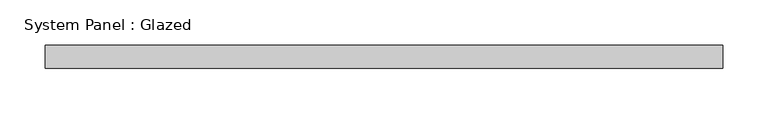
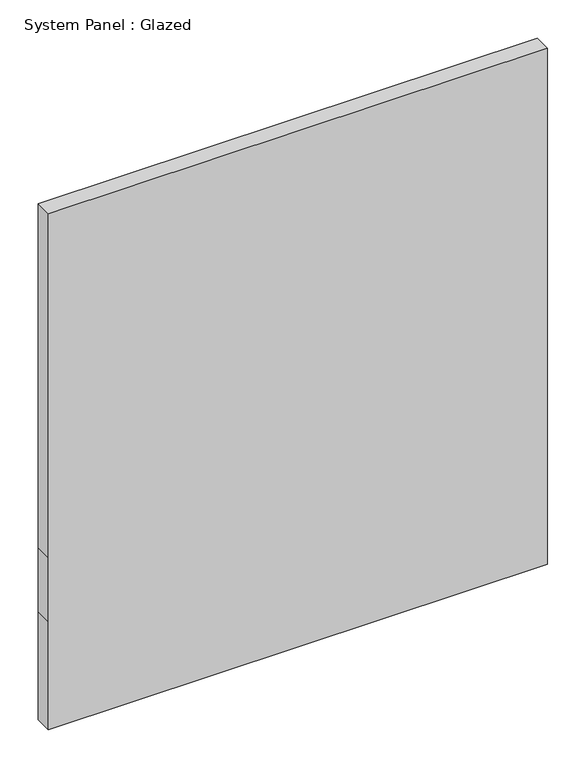
"""IFC4 building model written with IfcOpenShell, lengths in millimetres: plate geometry, System Panel : Glazed."""

from ifc_helpers import new_model, si_unit, frame, origin, place, context, project, spatial, polyline, outline, extrude, source, transform, mapped, element, save


def system_panel_glazed_e6cace74(model_context):
    return source(origin(), model_context, "Body", "SweptSolid", [
        extrude(outline(polyline([(0.0, -374.65), (0.0, 374.65), (171.3165682, 374.65), (272.8498523, 374.65), (818.549557, 374.65), (818.549557, -374.65), (272.8498523, -374.65), (171.3165682, -374.65), (0.0, -374.65)])), frame((0.0, 19.05, 0.0), z_axis=(0.0, 1.0, 0.0), x_axis=(0.0, 0.0, 1.0)), (0.0, 0.0, 1.0), 25.4),
    ])


if __name__ == "__main__":
    model = new_model("IFC4")
    model_context = context("Model", 3, world=origin())
    ifc_project = project(units=[si_unit("LENGTHUNIT", "METRE", prefix="MILLI")], contexts=[model_context])
    site = spatial("IfcSite", under=ifc_project)
    building = spatial("IfcBuilding", under=site)
    placement = place(None, origin())
    system_panel_glazed_shape = system_panel_glazed_e6cace74(model_context)
    element("IfcPlate", 1, ObjectType="System Panel : Glazed", at=placement, inside=building, context=model_context, shape_type="MappedRepresentation", body=[
        mapped(system_panel_glazed_shape, transform((0.0, 0.0, 0.0), x_axis=(1.0, 0.0, 0.0), y_axis=(0.0, 1.0, 0.0), z_axis=(0.0, 0.0, 1.0))),
    ])
    save(model, "model.ifc")

# Revit data of these elements
# Type "System Panel : Glazed"
#   Construction Type Id = "GSP4R"
#   Analytic Construction = "1/8 in Pilkington single glazing"
#   Visual Light Transmittance = 0.9
#   Solar Heat Gain Coefficient = 0.86
#   Heat Transfer Coefficient (U) = 1.18115 BTU/(h·ft²·°F)
#   Define Thermal Properties by = 1
# Element 1 (IfcPlate, "System Panel : Glazed")
#   Materials on its faces: "Glass"
# Materials
#   "Glass": class "Glass", colour RGB 0 128 192, transparency 0.75, Description = "Soda Lime Glass", Cost = 0
